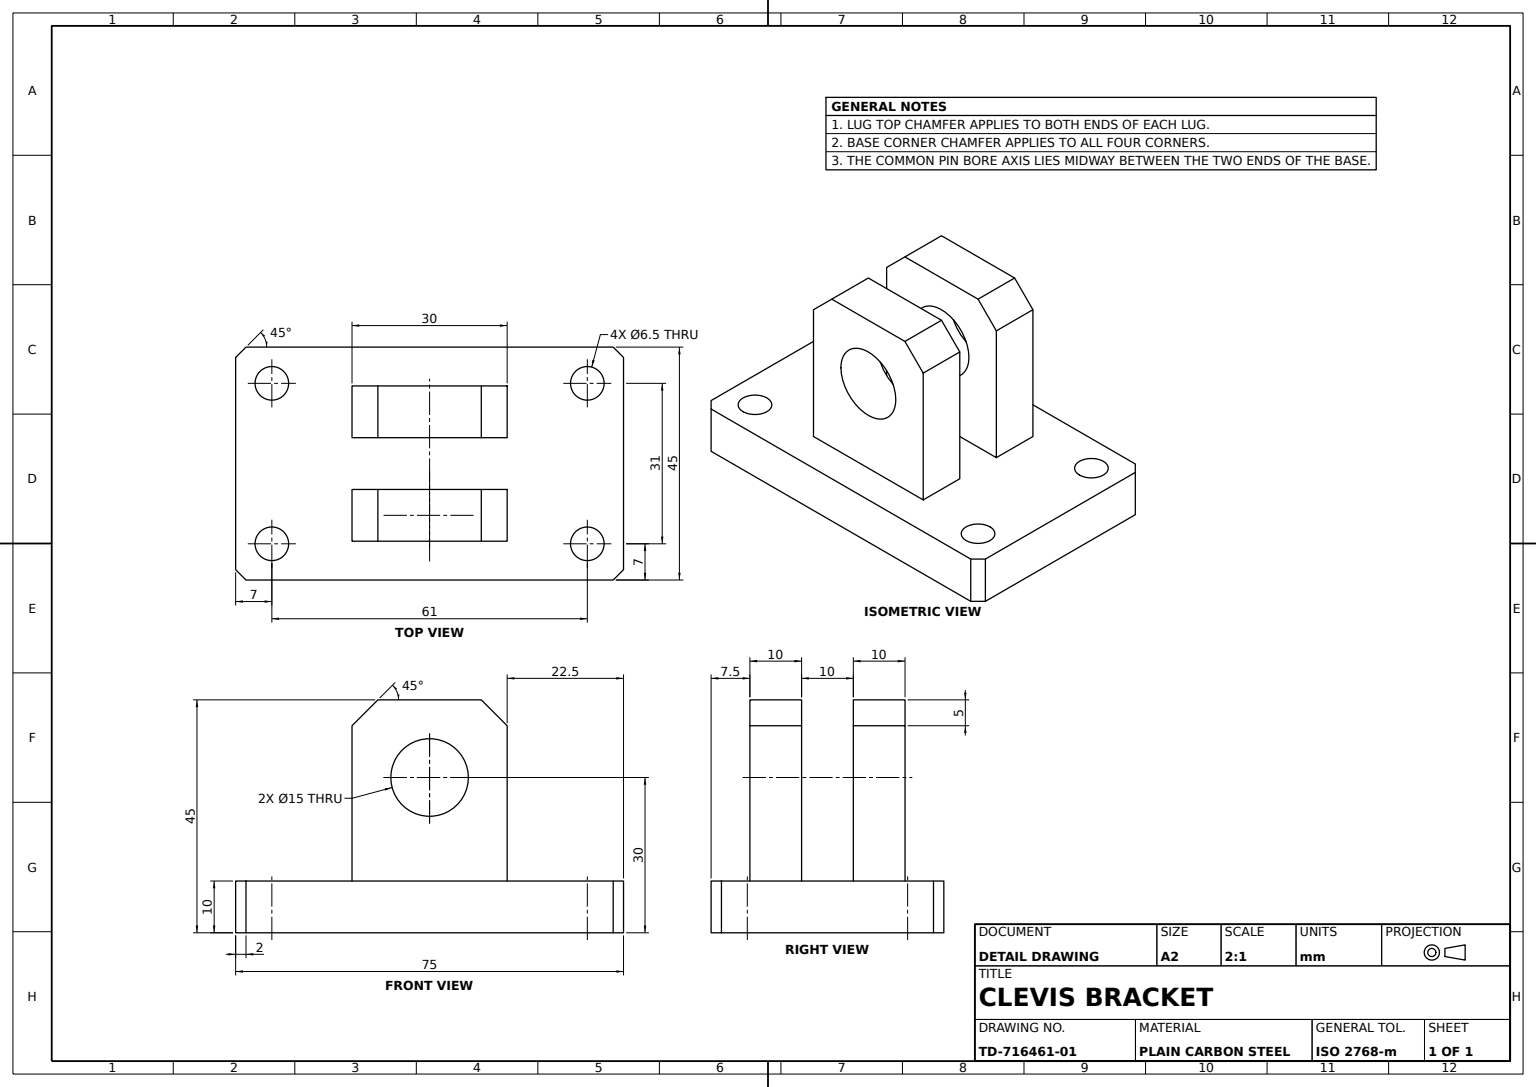
SolidWorks part; units mm, degrees
material "Plain Carbon Steel"
ref_plane "Front Plane" through (0, 0, 0) normal (0, 0, 1) x (1, 0, 0)
ref_plane "Top Plane" through (0, 0, 0) normal (0, 1, 0) x (1, 0, 0)
ref_plane "Right Plane" through (0, 0, 0) normal (1, 0, 0) x (0, 0, -1)
sketch "Base Plate Sketch" plane through (0, 0, 0) normal (0, 1, 0) x (1, 0, 0)
  line L1 (37.5, -22.5) -> (-37.5, -22.5)
  line L2 (37.5, -22.5) -> (37.5, 22.5)
  line L3 (37.5, 22.5) -> (-37.5, 22.5)
  line L4 (-37.5, -22.5) -> (-37.5, 22.5)
  line L5 (37.5, -22.5) -> (-37.5, 22.5) construction
  line L6 (37.5, 22.5) -> (-37.5, -22.5) construction
  point P0 (0, 0)
  dimension "D1" = 75
  dimension "D2" = 45
extrude "Base Plate 75x45x10" add sketch "Base Plate Sketch" along normal blind 10
sketch "Lug Profile Sketch" plane through (0, 10, 0) normal (0, 1, 0) x (1, 0, 0)
  line L0 (-37.5, -22.5) -> (37.5, -22.5) construction
  line L1 (-15, -15) -> (15, -15)
  line L2 (-15, -15) -> (-15, -5)
  line L3 (-15, -5) -> (15, -5)
  line L4 (15, -15) -> (15, -5)
  line L5 (-15, -15) -> (15, -5) construction
  line L6 (-15, -5) -> (15, -15) construction
  point P0 (0, -10)
  dimension "D1" = 7.5
  dimension "D2" = 10
  dimension "D3" = 30
extrude "Clevis Lug" add sketch "Lug Profile Sketch" along normal blind 35
mirror "Clevis Lug Mirror" about plane through (0, 0, 0) normal (0, 0, 1) of "Clevis Lug"
chamfer "Lug Top Chamfers 5mm" distance 5 angle 45 4 edges at (-15, 45, 10) (-15, 45, -10) (15, 45, -10) (15, 45, 10)
chamfer "Base Plate Edge Chamfer 2mm" distance 2 angle 45 4 edges at (-37.5, 5, 22.5) (-37.5, 5, -22.5) (37.5, 5, -22.5) (37.5, 5, 22.5)
sketch "Mounting Hole Sketch" plane through (0, 10, 0) normal (0, 1, 0) x (1, 0, 0)
  circle A0 centre (-30.5, 15.5) radius 3.25
  dimension "D2" = 6.5
  dimension "D1" = 30.5
  dimension "D3" = 15.5
extrude "Mounting Hole Ø6.5" cut sketch "Mounting Hole Sketch" against normal through all
mirror "Mounting Hole Mirror Front" about plane through (0, 0, 0) normal (0, 0, 1) of "Mounting Hole Ø6.5"
mirror "Mounting Holes Mirror Right" about plane through (0, 0, 0) normal (1, 0, 0) of "Mounting Hole Mirror Front", "Mounting Hole Ø6.5"
sketch "Pin Bore Sketch" plane through (0, 0, 15) normal (0, 0, 1) x (1, 0, 0)
  circle A0 centre (0, 30) radius 7.5
  dimension "D1" = 15
  dimension "D2" = 30
extrude "Pin Bore Ø15" cut sketch "Pin Bore Sketch" against normal through all
